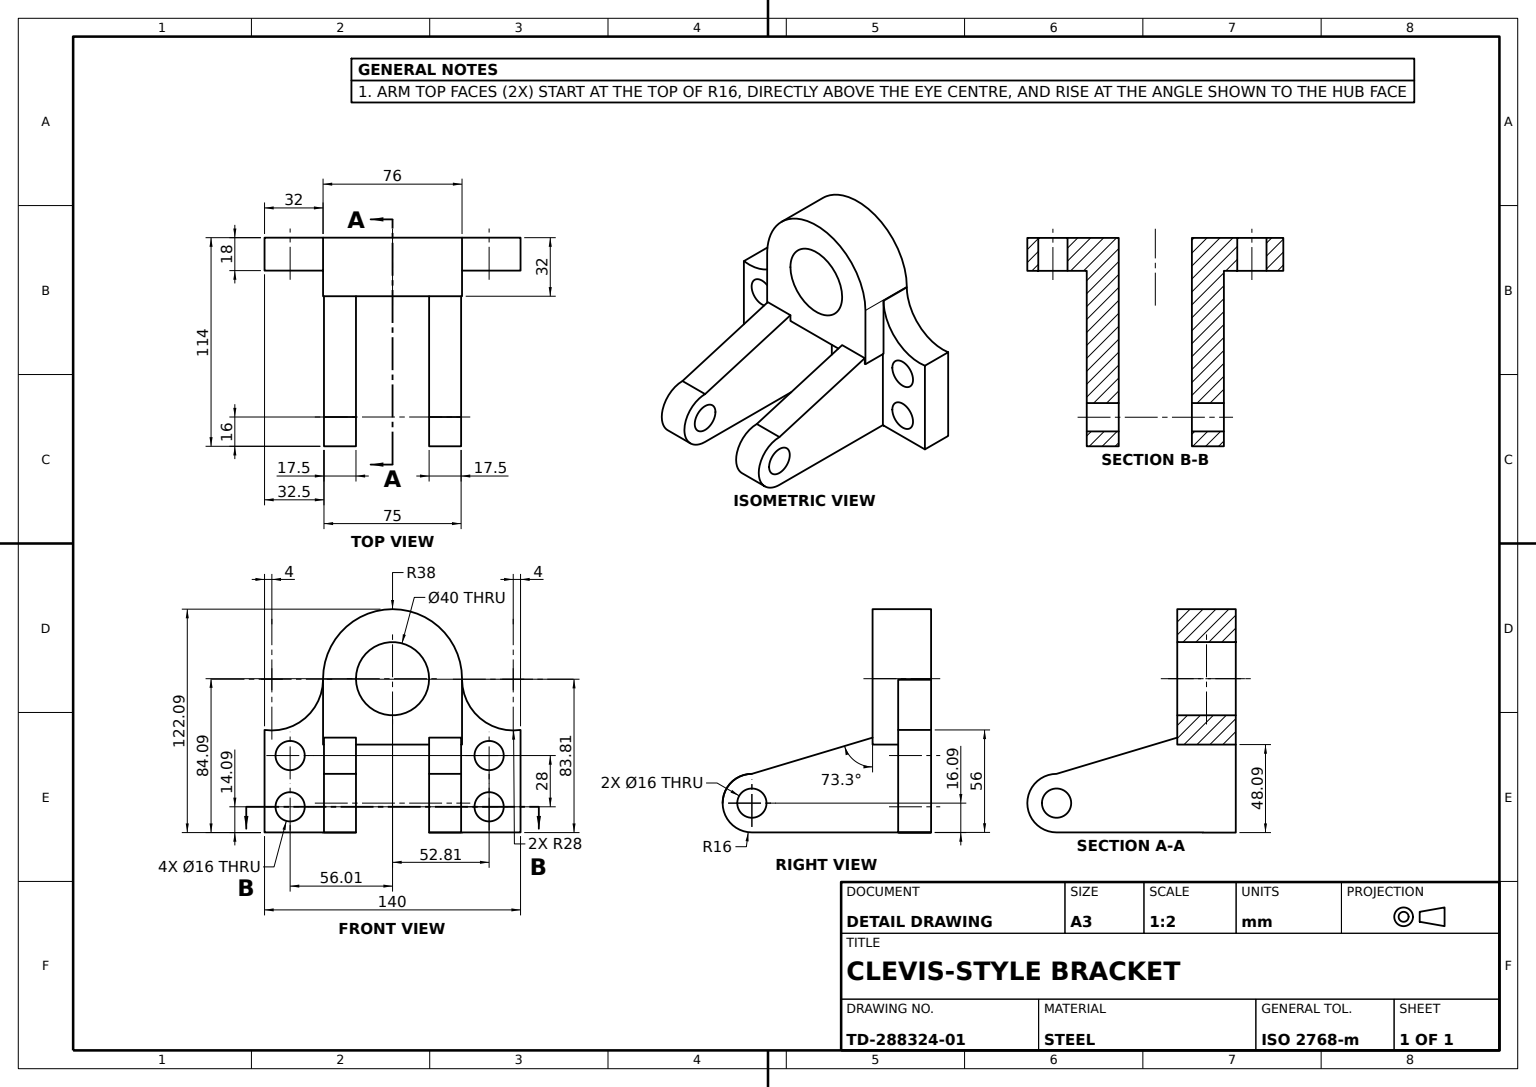
from build123d import *

# Parameters (mm, degrees)
HUB_BODY_SKETCH_R             = 20
HUB_BODY_DEPTH                = 32
MOUNTING_PLATE_DEPTH          = 18
SIDE_WEB_SKETCH_W             = 18
SIDE_WEB_SKETCH_H             = 48.092935693
SIDE_WEB_DEPTH                = 18
FORK_ARMS_DEPTH               = 37.5
FORK_SLOT_SKETCH_W            = 40
FORK_SLOT_SKETCH_H            = 48
FORK_SLOT_DEPTH               = 140.971425655
HUB_RELIEF_CUT_DEPTH          = 153.87903715
FORK_PIN_HOLE_SKETCH_R        = 8
FORK_PIN_HOLE_16_DEPTH        = 174.286612293
PLATE_MOUNTING_HOLES_SKETCH_R = 8
PLATE_MOUNTING_HOLES_16_DEPTH = 140.971425655


with BuildPart() as part:
    # Hub Body Sketch → Hub Body (new body)
    with BuildSketch(Plane.XY):
        with BuildLine():
            Line((-38, 36), (-38, 0))
            Line((-38, 0), (38, 0))
            Line((38, 0), (38, 36))
            ThreePointArc((38, 36), (0, 74), (-38, 36))
        make_face()
        with Locations((0, 36)):
            Circle(HUB_BODY_SKETCH_R, mode=Mode.SUBTRACT)
    extrude(amount=HUB_BODY_DEPTH)

    # Mounting Plate Sketch → Mounting Plate (add)
    with BuildSketch(Plane.XY):
        with BuildLine():
            Line((-38, -48), (-38, 35.425199961))
            ThreePointArc((-38, 35.425199961), (-47.777657825, 14.452308355), (-70, 8))
            Line((-70, 8), (-70, -48))
            Line((-70, -48), (-38, -48))
        make_face()
        with BuildLine():
            ThreePointArc((70, 8), (47.777657825, 14.452308355), (38, 35.425199961))
            Line((38, 35.425199961), (38, -48))
            Line((38, -48), (70, -48))
            Line((70, -48), (70, 8))
        make_face()
    extrude(amount=MOUNTING_PLATE_DEPTH)

    # Side Web Sketch → Side Web (add)
    with BuildSketch(Plane.XY):
        with Locations((-29, -24.046467847)):
            Rectangle(SIDE_WEB_SKETCH_W, SIDE_WEB_SKETCH_H)
        with Locations((29, -24.046467847)):
            Rectangle(SIDE_WEB_SKETCH_W, SIDE_WEB_SKETCH_H)
    extrude(amount=SIDE_WEB_DEPTH)

    # Fork Arms Sketch → Fork Arms (add, symmetric)
    with BuildSketch(Plane(origin=(0, 0, 0), x_dir=(0, 0, -1), z_dir=(1, 0, 0))):
        with BuildLine():
            Line((-98, -48), (-18, -48))
            Line((-18, -48), (-18, 8))
            Line((-18, 8), (-98, -16))
            ThreePointArc((-98, -16), (-114, -32), (-98, -48))
        make_face()
    extrude(amount=FORK_ARMS_DEPTH, both=True)

    # Fork Slot Sketch → Fork Slot (cut, through all)
    with BuildSketch(Plane(origin=(0, 0, 18), x_dir=(-1, 0, 0), z_dir=(0, 0, -1))):
        with Locations((0, -24)):
            Rectangle(FORK_SLOT_SKETCH_W, FORK_SLOT_SKETCH_H)
    extrude(amount=-FORK_SLOT_DEPTH, mode=Mode.SUBTRACT)

    # Hub Relief Sketch → Hub Relief Cut (cut, through all)
    with BuildSketch(Plane(origin=(0, 0, 0), x_dir=(-1, 0, 0), z_dir=(0, -1, 0))):
        Polygon((-20, -44.666666667), (20, -44.666666667), (20, -32), (11.078422409, -32), (-20, -32), align=None)
    extrude(amount=-HUB_RELIEF_CUT_DEPTH, mode=Mode.SUBTRACT)

    # Fork Pin Hole Sketch → Fork Pin Hole Ø16 (cut, through all)
    with BuildSketch(Plane.ZY.offset(37.5)):
        with Locations((98, -32)):
            Circle(FORK_PIN_HOLE_SKETCH_R)
    extrude(amount=-FORK_PIN_HOLE_16_DEPTH, mode=Mode.SUBTRACT)

    # Plate Mounting Holes Sketch → Plate Mounting Holes Ø16 (cut, through all)
    with BuildSketch(Plane.XY.offset(18)):
        with Locations((-56.00649608, -6)):
            Circle(PLATE_MOUNTING_HOLES_SKETCH_R)
        with Locations((-56.00649608, -34)):
            Circle(PLATE_MOUNTING_HOLES_SKETCH_R)
        with Locations((52.812642943, -6)):
            Circle(PLATE_MOUNTING_HOLES_SKETCH_R)
        with Locations((52.812642943, -34)):
            Circle(PLATE_MOUNTING_HOLES_SKETCH_R)
    extrude(amount=-PLATE_MOUNTING_HOLES_16_DEPTH, mode=Mode.SUBTRACT)


solid = part.part
